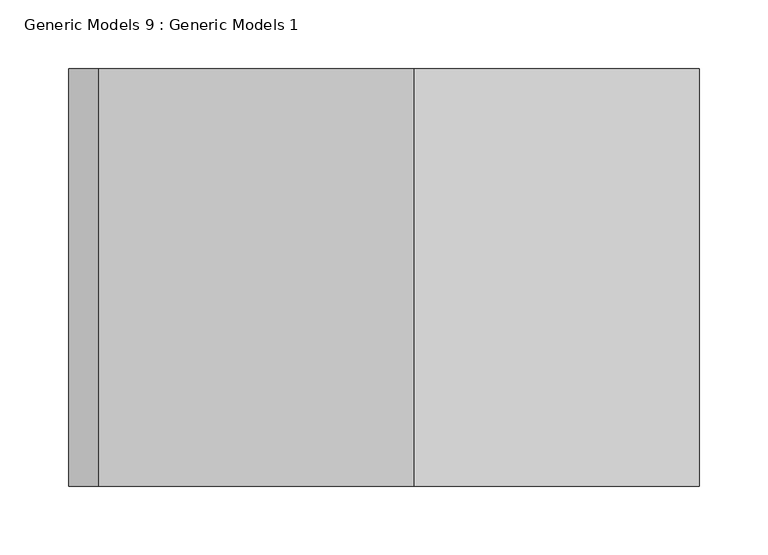
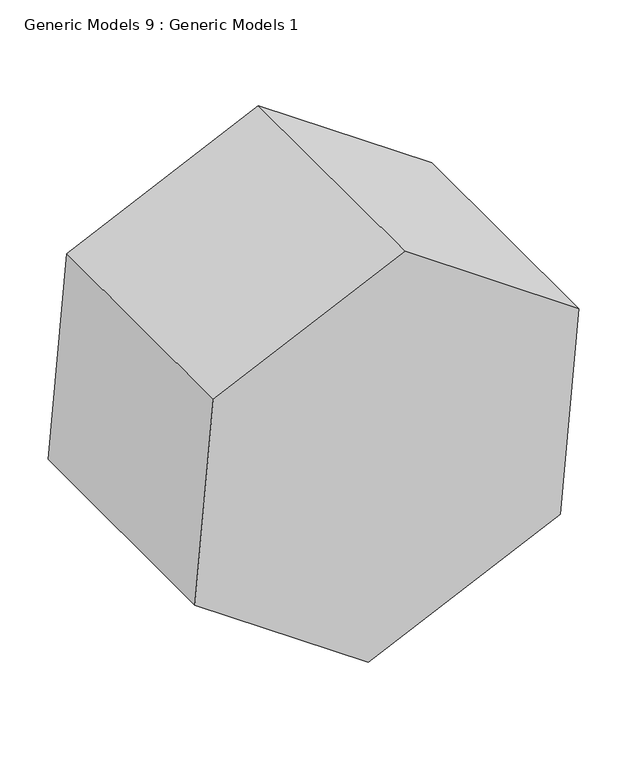
"""IFC4 building model written with IfcOpenShell, lengths in millimetres: proxy geometry, Generic Models 9 : Generic Models 1."""

from ifc_helpers import new_model, si_unit, frame, origin, place, context, project, spatial, polyline, outline, extrude, source, transform, mapped, element, save


def generic_models_9_generic_models_1_6881e9d4(model_context):
    return source(origin(), model_context, "Body", "SweptSolid", [
        extrude(outline(polyline([(833.1013393, 1418.8920945), (978.7897542, 1210.8274753), (871.4447157, 980.6252974), (618.4112624, 958.4877387), (472.7228475, 1166.552358), (580.067886, 1396.7545359), (833.1013393, 1418.8920945)])), frame((0.0, -10720.3372434, 0.0), z_axis=(0.0, 1.0, 0.0), x_axis=(0.0, 0.0, 1.0)), (0.0, 0.0, 1.0), 304.8),
    ])


if __name__ == "__main__":
    model = new_model("IFC4")
    model_context = context("Model", 3, world=origin())
    ifc_project = project(units=[si_unit("LENGTHUNIT", "METRE", prefix="MILLI")], contexts=[model_context])
    site = spatial("IfcSite", under=ifc_project)
    building = spatial("IfcBuilding", under=site)
    placement = place(None, origin())
    generic_models_9_generic_models_1_shape = generic_models_9_generic_models_1_6881e9d4(model_context)
    element("IfcBuildingElementProxy", 1, Name="Generic Models 9 : Generic Models 1", ObjectType="Generic Models 9 : Generic Models 1", at=placement, inside=building, context=model_context, shape_type="MappedRepresentation", body=[
        mapped(generic_models_9_generic_models_1_shape, transform((0.0, 0.0, 0.0), x_axis=(1.0, 0.0, 0.0), y_axis=(0.0, 1.0, 0.0), z_axis=(0.0, 0.0, 1.0))),
    ])
    save(model, "model.ifc")
